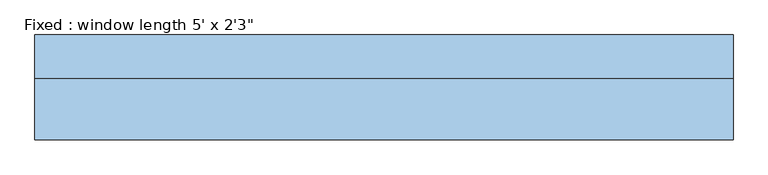
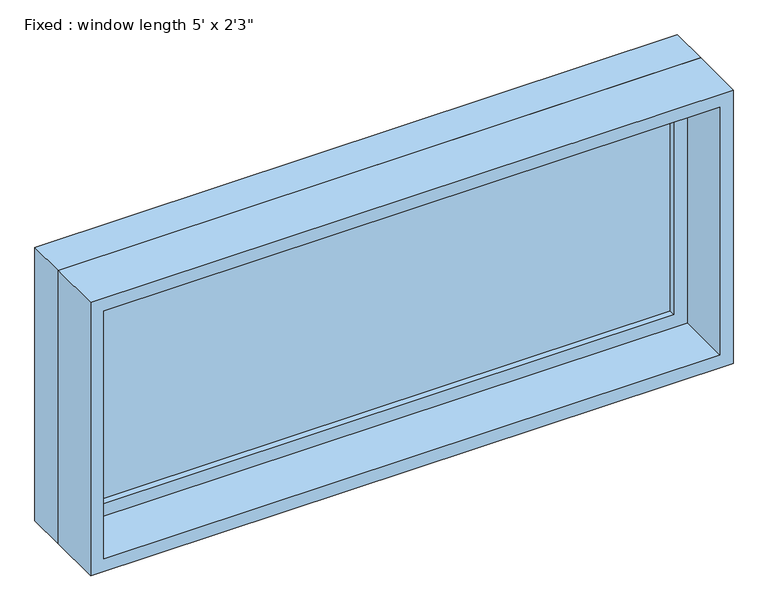
"""IFC4 building model written with IfcOpenShell, lengths in millimetres: window geometry."""

from ifc_helpers import new_model, si_unit, frame, origin, place, context, project, spatial, polyline, outline, extrude, source, transform, mapped, element, save


def window_e88f44c6(model_context):
    return source(origin(), model_context, "Body", "SweptSolid", [
        extrude(outline(polyline([(660.4, 34.925), (-736.6, 34.925), (-736.6, 47.625), (660.4, 47.625), (660.4, 34.925)])), frame((0.0, 0.0, 977.9), z_axis=(0.0, 0.0, 1.0), x_axis=(1.0, 0.0, 0.0)), (0.0, 0.0, 1.0), 558.8),
        extrude(outline(polyline([(1581.15, -781.05), (933.45, -781.05), (933.45, 704.85), (1581.15, 704.85), (1581.15, -781.05)]), holes=[polyline([(1536.7, -736.6), (1536.7, 660.4), (977.9, 660.4), (977.9, -736.6), (1536.7, -736.6)])]), frame((0.0, 19.05, 0.0), z_axis=(0.0, 1.0, 0.0), x_axis=(0.0, 0.0, 1.0)), (0.0, 0.0, 1.0), 44.45),
        extrude(outline(polyline([(1600.2, -800.1), (914.4, -800.1), (914.4, 723.9), (1600.2, 723.9), (1600.2, -800.1)]), holes=[polyline([(1568.45, -768.35), (1568.45, 692.15), (946.15, 692.15), (946.15, -768.35), (1568.45, -768.35)])]), frame((0.0, -114.3, 0.0), z_axis=(0.0, 1.0, 0.0), x_axis=(0.0, 0.0, 1.0)), (0.0, 0.0, 1.0), 133.35),
        extrude(outline(polyline([(1600.2, 723.9), (1600.2, -800.1), (914.4, -800.1), (914.4, 723.9), (1600.2, 723.9)]), holes=[polyline([(1581.15, 704.85), (933.45, 704.85), (933.45, -781.05), (1581.15, -781.05), (1581.15, 704.85)])]), frame((0.0, 19.05, 0.0), z_axis=(0.0, 1.0, 0.0), x_axis=(0.0, 0.0, 1.0)), (0.0, 0.0, 1.0), 95.25),
    ])


if __name__ == "__main__":
    model = new_model("IFC4")
    model_context = context("Model", 3, world=origin())
    ifc_project = project(units=[si_unit("LENGTHUNIT", "METRE", prefix="MILLI")], contexts=[model_context])
    site = spatial("IfcSite", under=ifc_project)
    building = spatial("IfcBuilding", under=site)
    placement = place(None, origin())
    window_shape = window_e88f44c6(model_context)
    element("IfcWindow", 1, ObjectType="Fixed : window length 5' x 2'3\"", at=placement, inside=building, context=model_context, shape_type="MappedRepresentation", body=[
        mapped(window_shape, transform((0.0, 0.0, 0.0), x_axis=(1.0, 0.0, 0.0), y_axis=(0.0, 1.0, 0.0), z_axis=(0.0, 0.0, 1.0))),
    ])
    save(model, "model.ifc")

# Revit data of these elements
# Type "Fixed : window length 5' x 2'3\""
#   Type Mark = "28"
#   Construction Type Id = "GSP4R"
#   Assembly Code = "B2020100"
#   Analytic Construction = "1/8 in Pilkington single glazing"
#   Visual Light Transmittance = 0.9
#   Solar Heat Gain Coefficient = 0.78
#   Heat Transfer Coefficient (U) = 0.6496 BTU/(h·ft²·°F)
#   Height = 2' - 3"
#   Default Sill Height = 3' - 0"
#   Width = 5' - 0"
#   Window Inset = 0' - 2"
#   Define Thermal Properties by = 1
#   Glass Pane Material = Glass
#   Sash Material = Sash
#   Wall Closure = (empty or 0)
# Element 1 (IfcWindow, "Fixed : window length 5' x 2'3\"")
#   Materials on its faces: "Sash", "Glass"
# Materials
#   "Glass": class "Glass", colour RGB 0 128 192, transparency 0.75, Description = "Soda Lime Glass", Cost = 0
#   "Sash": class "Wood", colour RGB 224 178 126, transparency 0, Cost = 0
